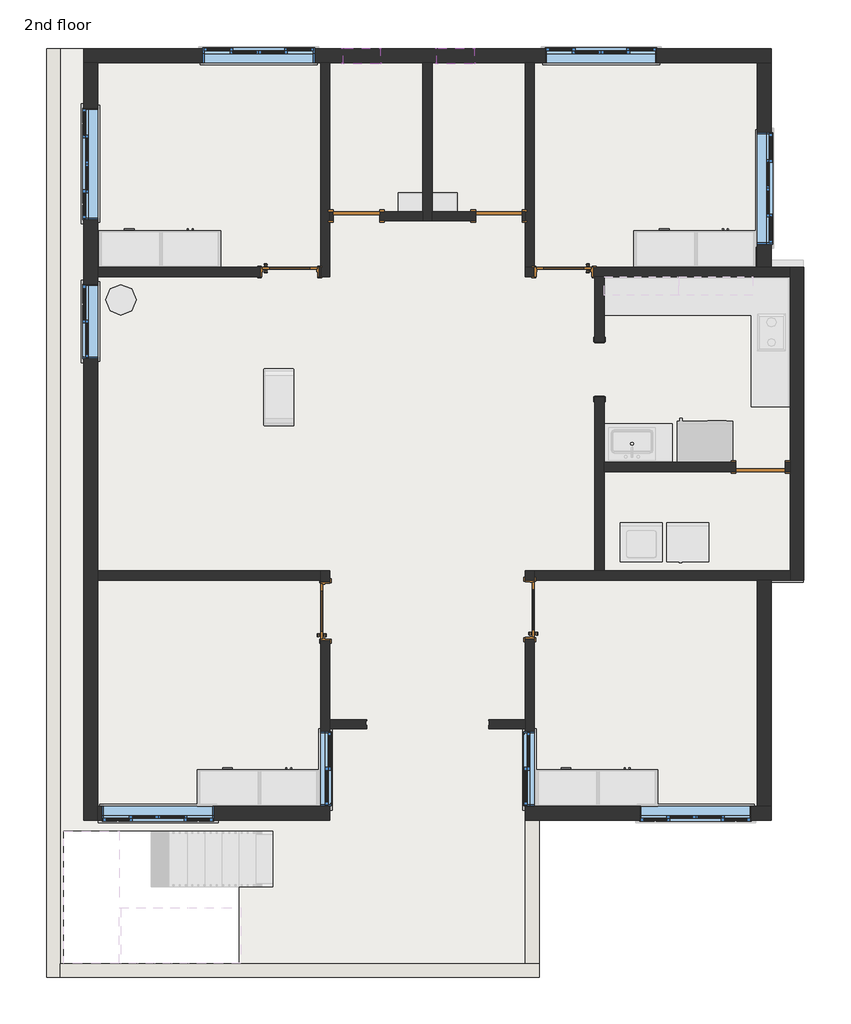
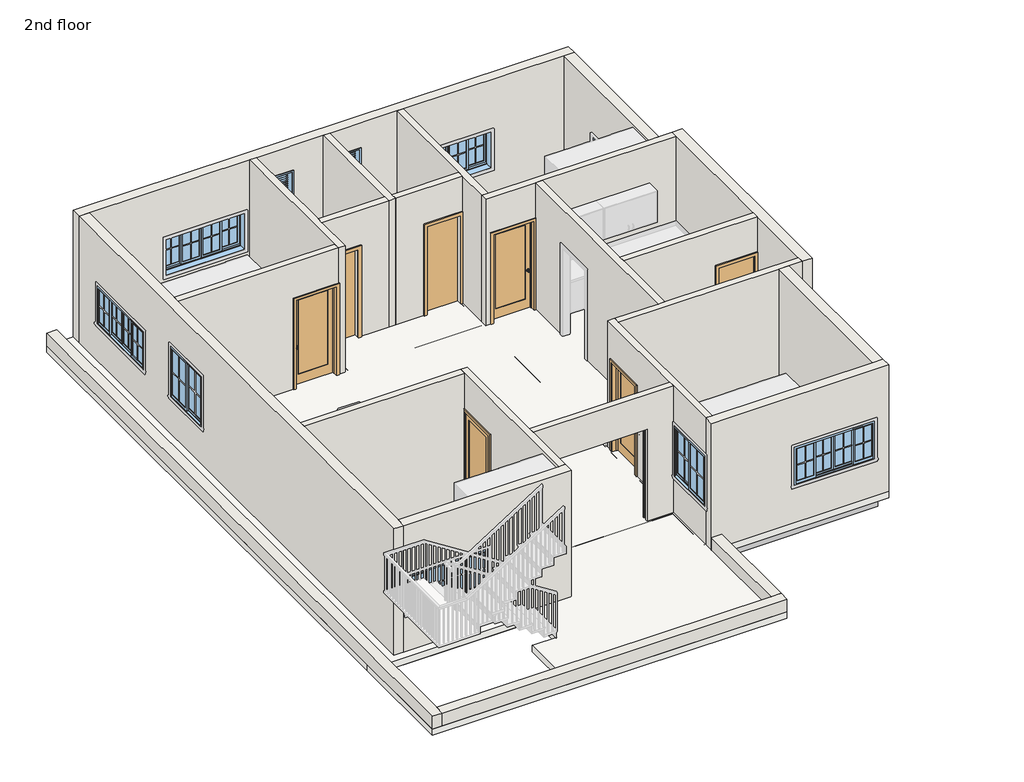
# One storey, part 1 of 4: 24 walls, 11 windows, 7 beams, 7 doors, 1 slab.
"""IFC4 building model written with IfcOpenShell, lengths in millimetres."""

from ifc_helpers import new_model, si_unit, frame, origin, place, context, project, spatial, polyline, outline, extrude, faceted_brep, transform, mapped, element, save
from components import door_010cc4d9, door_5a860750, door_e2b13fe9, door_a9addea7, door_bb092f7c, window_f2d8fef0, window_c1e3dfc0, window_49fe3060, window_58cce754

model = new_model("IFC4")

# Units and contexts
model_context = context("Model", 3, world=origin())
ifc_project = project(units=[si_unit("LENGTHUNIT", "METRE", prefix="MILLI")], contexts=[model_context])

# Site, building, storey
site = spatial("IfcSite", under=ifc_project)
building = spatial("IfcBuilding", under=site)
storey = spatial("IfcBuildingStorey", under=building, Name="2nd floor", Elevation=7010.4)

# Beams
placement = place(None, origin())
element("IfcBeam", 1, ObjectType="Concrete-Rectangular Beam", at=placement, inside=storey, context=model_context, shape_type="SweptSolid", body=[
    extrude(outline(polyline([(-1593.2124084, 1316.1961804), (-1364.6124084, 1316.1961804), (-1364.6124084, -2163.6038196), (-1593.2124084, -2163.6038196), (-1593.2124084, 1316.1961804)])), frame((0.0, 0.0, 6705.6), z_axis=(0.0, 0.0, 1.0), x_axis=(1.0, 0.0, 0.0)), (0.0, 0.0, 1.0), 304.8),
])
element("IfcBeam", 2, ObjectType="Concrete-Rectangular Beam", at=placement, inside=storey, context=model_context, shape_type="Brep", body=[
    faceted_brep([(-1593.2124084, -2201.7038196, 7010.4), (-5212.7124084, -2201.7038196, 7010.4), (-5441.3124084, -2201.7038196, 7010.4), (-5441.3124084, -2239.8038196, 7010.4), (-5174.6124084, -2239.8038196, 7010.4), (-5174.6124084, -2430.3038196, 7010.4), (-1593.2124084, -2430.3038196, 7010.4), (-1593.2124084, -2201.7038196, 6705.6), (-5212.7124084, -2201.7038196, 6705.6), (-5441.3124084, -2201.7038196, 6705.6), (-1593.2124084, -2430.3038196, 6705.6), (-5174.6124084, -2430.3038196, 6705.6), (-5174.6124084, -2239.8038196, 6705.6), (-5441.3124084, -2239.8038196, 6705.6)], [[[0, 1, 2, 3, 4, 5, 6]], [[0, 7, 8, 9, 2, 1]], [[9, 8, 7, 10, 11, 12, 13]], [[10, 6, 5, 11]], [[7, 0, 6, 10]], [[2, 9, 13, 3]], [[12, 4, 3, 13]], [[4, 12, 11, 5]]]),
])
element("IfcBeam", 3, ObjectType="Concrete-Rectangular Beam", at=placement, inside=storey, context=model_context, shape_type="Brep", body=[
    faceted_brep([(-8756.0124084, -2468.4038196, 7010.4), (-8756.0124084, -2239.8038196, 7010.4), (-8794.1124084, -2239.8038196, 7010.4), (-12413.6124084, -2239.8038196, 7010.4), (-12413.6124084, -2468.4038196, 7010.4), (-8756.0124084, -2239.8038196, 6705.6), (-8794.1124084, -2239.8038196, 6705.6), (-12413.6124084, -2239.8038196, 6705.6), (-8756.0124084, -2468.4038196, 6705.6), (-12413.6124084, -2468.4038196, 6705.6)], [[[0, 1, 2, 3, 4]], [[1, 5, 6, 7, 3, 2]], [[5, 8, 9, 7, 6]], [[8, 0, 4, 9]], [[1, 0, 8, 5]], [[4, 3, 7, 9]]]),
])
element("IfcBeam", 4, ObjectType="Concrete-Rectangular Beam", at=placement, inside=storey, context=model_context, shape_type="SweptSolid", body=[
    extrude(outline(polyline([(-12642.2124084, 9875.9961804), (-12413.6124084, 9875.9961804), (-12413.6124084, 6751.7961804), (-12642.2124084, 6751.7961804), (-12642.2124084, 9875.9961804)])), frame((0.0, 0.0, 6705.6), z_axis=(0.0, 0.0, 1.0), x_axis=(1.0, 0.0, 0.0)), (0.0, 0.0, 1.0), 304.8),
    extrude(outline(polyline([(-12413.6124084, -2163.6038196), (-12642.2124084, -2163.6038196), (-12642.2124084, 1392.3961804), (-12413.6124084, 1392.3961804), (-12413.6124084, -2163.6038196)])), frame((0.0, 0.0, 6705.6), z_axis=(0.0, 0.0, 1.0), x_axis=(1.0, 0.0, 0.0)), (0.0, 0.0, 1.0), 304.8),
    extrude(outline(polyline([(-12413.6124084, 1697.1961804), (-12642.2124084, 1697.1961804), (-12642.2124084, 6446.9961804), (-12413.6124084, 6446.9961804), (-12413.6124084, 1697.1961804)])), frame((0.0, 0.0, 6705.6), z_axis=(0.0, 0.0, 1.0), x_axis=(1.0, 0.0, 0.0)), (0.0, 0.0, 1.0), 304.8),
])
element("IfcBeam", 5, ObjectType="Concrete-Rectangular Beam", at=placement, inside=storey, context=model_context, shape_type="Brep", body=[
    faceted_brep([(-843.9124084, 1659.0961804, 7010.4), (-843.9124084, 1430.4961804, 7010.4), (-843.9124084, 1430.4961804, 6705.6), (-843.9124084, 1659.0961804, 6705.6), (-5098.4124084, 1659.0961804, 7010.4), (-5098.4124084, 1468.5961804, 7010.4), (-5403.2124084, 1468.5961804, 7010.4), (-5403.2124084, 1659.0961804, 7010.4), (-5441.3124084, 1659.0961804, 7010.4), (-8565.5124084, 1659.0961804, 7010.4), (-8603.6124084, 1659.0961804, 7010.4), (-8603.6124084, 1468.5961804, 7010.4), (-8908.4124084, 1468.5961804, 7010.4), (-8908.4124084, 1659.0961804, 7010.4), (-12413.6124084, 1659.0961804, 7010.4), (-12413.6124084, 1430.4961804, 7010.4), (-8794.1124084, 1430.4961804, 7010.4), (-8565.5124084, 1430.4961804, 7010.4), (-5441.3124084, 1430.4961804, 7010.4), (-5212.7124084, 1430.4961804, 7010.4), (-1593.2124084, 1430.4961804, 7010.4), (-1593.2124084, 1620.9961804, 7010.4), (-1364.6124084, 1620.9961804, 7010.4), (-1364.6124084, 1430.4961804, 7010.4), (-1364.6124084, 1430.4961804, 6705.6), (-1364.6124084, 1620.9961804, 6705.6), (-1593.2124084, 1620.9961804, 6705.6), (-1593.2124084, 1430.4961804, 6705.6), (-5212.7124084, 1430.4961804, 6705.6), (-5441.3124084, 1430.4961804, 6705.6), (-8565.5124084, 1430.4961804, 6705.6), (-8794.1124084, 1430.4961804, 6705.6), (-12413.6124084, 1430.4961804, 6705.6), (-12413.6124084, 1659.0961804, 6705.6), (-8908.4124084, 1659.0961804, 6705.6), (-8908.4124084, 1468.5961804, 6705.6), (-8603.6124084, 1468.5961804, 6705.6), (-8603.6124084, 1659.0961804, 6705.6), (-8565.5124084, 1659.0961804, 6705.6), (-5441.3124084, 1659.0961804, 6705.6), (-5403.2124084, 1659.0961804, 6705.6), (-5403.2124084, 1468.5961804, 6705.6), (-5098.4124084, 1468.5961804, 6705.6), (-5098.4124084, 1659.0961804, 6705.6)], [[[0, 1, 2, 3]], [[1, 0, 4, 5, 6, 7, 8, 9, 10, 11, 12, 13, 14, 15, 16, 17, 18, 19, 20, 21, 22, 23]], [[2, 1, 23, 24]], [[3, 2, 24, 25, 26, 27, 28, 29, 30, 31, 32, 33, 34, 35, 36, 37, 38, 39, 40, 41, 42, 43]], [[0, 3, 43, 4]], [[15, 14, 33, 32]], [[22, 25, 24, 23]], [[26, 21, 20, 27]], [[21, 26, 25, 22]], [[15, 32, 31, 30, 29, 28, 27, 20, 19, 18, 17, 16]], [[36, 11, 10, 37]], [[11, 36, 35, 12]], [[12, 35, 34, 13]], [[33, 14, 13, 34]], [[42, 5, 4, 43]], [[5, 42, 41, 6]], [[6, 41, 40, 7]], [[37, 10, 9, 8, 7, 40, 39, 38]]]),
])
element("IfcBeam", 6, ObjectType="Concrete-Rectangular Beam", at=placement, inside=storey, context=model_context, shape_type="Brep", body=[
    faceted_brep([(-8794.1124084, -2239.8038196, 7010.4), (-8756.0124084, -2239.8038196, 7010.4), (-8565.5124084, -2239.8038196, 7010.4), (-8565.5124084, -1007.9038196, 7010.4), (-8565.5124084, -779.3038196, 7010.4), (-8565.5124084, 1430.4961804, 7010.4), (-8794.1124084, 1430.4961804, 7010.4), (-8794.1124084, -2239.8038196, 6705.6), (-8794.1124084, 1430.4961804, 6705.6), (-8565.5124084, -2239.8038196, 6705.6), (-8756.0124084, -2239.8038196, 6705.6), (-8565.5124084, 1430.4961804, 6705.6), (-8565.5124084, -779.3038196, 6705.6), (-8565.5124084, -1007.9038196, 6705.6)], [[[0, 1, 2, 3, 4, 5, 6]], [[7, 0, 6, 8]], [[9, 10, 7, 8, 11, 12, 13]], [[11, 5, 4, 3, 2, 9, 13, 12]], [[2, 1, 0, 7, 10, 9]], [[5, 11, 8, 6]]]),
    faceted_brep([(-8794.1124084, 9914.0961804, 7010.4), (-8565.5124084, 9914.0961804, 7010.4), (-8565.5124084, 9914.0961804, 6705.6), (-8794.1124084, 9914.0961804, 6705.6), (-8794.1124084, 6713.6961804, 7010.4), (-8794.1124084, 6713.6961804, 6705.6), (-8756.0124084, 6713.6961804, 6705.6), (-8756.0124084, 6713.6961804, 7010.4), (-8756.0124084, 6751.7961804, 7010.4), (-8565.5124084, 6751.7961804, 7010.4), (-8565.5124084, 7323.2961804, 7010.4), (-8565.5124084, 7551.8961804, 7010.4), (-8565.5124084, 7551.8961804, 6705.6), (-8565.5124084, 7323.2961804, 6705.6), (-8565.5124084, 6751.7961804, 6705.6), (-8756.0124084, 6751.7961804, 6705.6)], [[[0, 1, 2, 3]], [[4, 5, 6, 7]], [[1, 0, 4, 7, 8, 9, 10, 11]], [[3, 2, 12, 13, 14, 15, 6, 5]], [[0, 3, 5, 4]], [[2, 1, 11, 10, 9, 14, 13, 12]], [[15, 8, 7, 6]], [[8, 15, 14, 9]]]),
    faceted_brep([(-8794.1124084, 6485.0961804, 6705.6), (-8794.1124084, 6485.0961804, 7010.4), (-8756.0124084, 6485.0961804, 7010.4), (-8756.0124084, 6485.0961804, 6705.6), (-8565.5124084, 1659.0961804, 6705.6), (-8565.5124084, 1659.0961804, 7010.4), (-8603.6124084, 1659.0961804, 7010.4), (-8603.6124084, 1659.0961804, 6705.6), (-8565.5124084, 6446.9961804, 6705.6), (-8565.5124084, 6446.9961804, 7010.4), (-8794.1124084, 1697.1961804, 7010.4), (-8603.6124084, 1697.1961804, 7010.4), (-8756.0124084, 6446.9961804, 7010.4), (-8794.1124084, 1697.1961804, 6705.6), (-8603.6124084, 1697.1961804, 6705.6), (-8756.0124084, 6446.9961804, 6705.6)], [[[0, 1, 2, 3]], [[4, 5, 6, 7]], [[5, 4, 8, 9]], [[2, 1, 10, 11, 6, 5, 9, 12]], [[1, 0, 13, 10]], [[8, 4, 7, 14, 13, 0, 3, 15]], [[15, 12, 9, 8]], [[12, 15, 3, 2]], [[14, 11, 10, 13]], [[11, 14, 7, 6]]]),
])
element("IfcBeam", 7, ObjectType="Concrete-Rectangular Beam", at=placement, inside=storey, context=model_context, shape_type="SweptSolid", body=[
    extrude(outline(polyline([(-5441.3124084, -779.3038196), (-5441.3124084, -1007.9038196), (-8565.5124084, -1007.9038196), (-8565.5124084, -779.3038196), (-5441.3124084, -779.3038196)])), frame((0.0, 0.0, 6705.6), z_axis=(0.0, 0.0, 1.0), x_axis=(1.0, 0.0, 0.0)), (0.0, 0.0, 1.0), 304.8),
])

# Doors
door_shape = door_010cc4d9(model_context)
element("IfcDoor", 8, ObjectType="Door-Interior-Single-1_Panel-Wood : 36\" x 84\"", at=placement, inside=storey, context=model_context, shape_type="MappedRepresentation", body=[
    mapped(door_shape, transform((-9264.0124084, 6526.3711804, 7010.4), x_axis=(1.0, 0.0, 0.0), y_axis=(0.0, 1.0, 0.0), z_axis=(0.0, 0.0, 1.0))),
])
element("IfcDoor", 9, ObjectType="Door-Interior-Single-1_Panel-Wood : 36\" x 84\"", at=placement, inside=storey, context=model_context, shape_type="MappedRepresentation", body=[
    mapped(door_shape, transform((-8682.9874084, 960.5961804, 7010.4), x_axis=(0.0, 1.0, 0.0), y_axis=(-1.0, 0.0, 0.0), z_axis=(0.0, 0.0, 1.0))),
])
door_2_shape = door_5a860750(model_context)
element("IfcDoor", 10, ObjectType="Door-Interior-Single-1_Panel-Wood : 36\" x 84\"", at=placement, inside=storey, context=model_context, shape_type="MappedRepresentation", body=[
    mapped(door_2_shape, transform((-4768.2124084, 6526.3711804, 7010.4), x_axis=(-1.0, 0.0, 0.0), y_axis=(0.0, -1.0, 0.0), z_axis=(0.0, 0.0, 1.0))),
])
element("IfcDoor", 11, ObjectType="Door-Interior-Single-1_Panel-Wood : 36\" x 84\"", at=placement, inside=storey, context=model_context, shape_type="MappedRepresentation", body=[
    mapped(door_2_shape, transform((-5323.8374084, 985.9961804, 7010.4), x_axis=(0.0, 1.0, 0.0), y_axis=(-1.0, 0.0, 0.0), z_axis=(0.0, 0.0, 1.0))),
])
door_3_shape = door_e2b13fe9(model_context)
element("IfcDoor", 12, ObjectType="Single-Flush : 30\" x 84\"", at=placement, inside=storey, context=model_context, shape_type="MappedRepresentation", body=[
    mapped(door_3_shape, transform((-8171.8124084, 7437.5961804, 7010.4), x_axis=(-1.0, 0.0, 0.0), y_axis=(0.0, -1.0, 0.0), z_axis=(0.0, 0.0, 1.0))),
])
door_4_shape = door_a9addea7(model_context)
element("IfcDoor", 13, ObjectType="Single-Flush : 30\" x 84\"", at=placement, inside=storey, context=model_context, shape_type="MappedRepresentation", body=[
    mapped(door_4_shape, transform((-5835.0124084, 7437.5961804, 7010.4), x_axis=(1.0, 0.0, 0.0), y_axis=(0.0, 1.0, 0.0), z_axis=(0.0, 0.0, 1.0))),
])
door_5_shape = door_bb092f7c(model_context)
element("IfcDoor", 14, ObjectType="Single-Flush : 32\" x 84\"", at=placement, inside=storey, context=model_context, shape_type="MappedRepresentation", body=[
    mapped(door_5_shape, transform((-1542.4124084, 3322.7961804, 7010.4), x_axis=(1.0, 0.0, 0.0), y_axis=(0.0, 1.0, 0.0), z_axis=(0.0, 0.0, 1.0))),
])

# Slab
element("IfcSlab", 15, ObjectType="Generic - 6\"", at=placement, inside=storey, context=model_context, shape_type="SweptSolid", body=[
    extrude(outline(polyline([(-1364.6124084, 10180.7961804), (-1364.6124084, 6599.3961804), (-831.2124084, 6599.3961804), (-831.2124084, 1468.5961804), (-1364.6124084, 1468.5961804), (-1364.6124084, -2468.4038196), (-5174.6124084, -2468.4038196), (-5174.6124084, -5046.5038196), (-13251.8124084, -5046.5038196), (-13251.8124084, -2468.4038196), (-13251.8124084, 10180.7961804), (-1364.6124084, 10180.7961804)]), holes=[polyline([(-9543.8120641, -3536.9669819), (-9543.8120641, -2647.9669819), (-12972.8120641, -2647.9669819), (-12972.8120641, -4817.9038196), (-10102.6120641, -4817.9038196), (-10102.6120641, -3536.9669819), (-9543.8120641, -3536.9669819)])]), frame((0.0, 0.0, 6858.0), z_axis=(0.0, 0.0, 1.0), x_axis=(1.0, 0.0, 0.0)), (0.0, 0.0, 1.0), 152.4),
])

# Walls
element("IfcWall", 16, ObjectType="Generic - 6\"", at=placement, inside=storey, context=model_context, shape_type="Brep", body=[
    faceted_brep([(-8756.0124084, 9952.1961804, 7010.4), (-8756.0124084, 6599.3961804, 7010.4), (-8756.0124084, 6446.9961804, 7010.4), (-8756.0124084, 6446.9961804, 10058.4), (-8756.0124084, 6599.3961804, 10058.4), (-8756.0124084, 9952.1961804, 10058.4), (-8603.6124084, 9952.1961804, 7010.4), (-8603.6124084, 9952.1961804, 10058.4), (-8603.6124084, 7513.7961804, 10058.4), (-8603.6124084, 7361.3961804, 10058.4), (-8603.6124084, 6446.9961804, 10058.4), (-8603.6124084, 6446.9961804, 7010.4), (-8603.6124084, 7361.3961804, 7010.4), (-8603.6124084, 7513.7961804, 7010.4)], [[[0, 1, 2, 3, 4, 5]], [[6, 7, 8, 9, 10, 11, 12, 13]], [[2, 1, 0, 6, 13, 12, 11]], [[0, 5, 7, 6]], [[3, 2, 11, 10]], [[5, 4, 3, 10, 9, 8, 7]]]),
])
element("IfcWall", 17, ObjectType="Generic - 6\"", at=placement, inside=storey, context=model_context, shape_type="SweptSolid", body=[
    extrude(outline(polyline([(7010.4, -8756.0124084), (10058.4, -8756.0124084), (10058.4, -12413.6124084), (7010.4, -12413.6124084), (7010.4, -9746.6124084), (9169.4, -9746.6124084), (9169.4, -8781.4124084), (7010.4, -8781.4124084), (7010.4, -8756.0124084)])), frame((0.0, 6446.9961804, 0.0), z_axis=(0.0, 1.0, 0.0), x_axis=(0.0, 0.0, 1.0)), (0.0, 0.0, 1.0), 152.4),
])
element("IfcWall", 18, ObjectType="Generic - 6\"", at=placement, inside=storey, context=model_context, shape_type="Brep", body=[
    faceted_brep([(-7079.6124084, 9952.1961804, 7010.4), (-7079.6124084, 7513.7961804, 7010.4), (-7079.6124084, 7361.3961804, 7010.4), (-7079.6124084, 7361.3961804, 10058.4), (-7079.6124084, 7513.7961804, 10058.4), (-7079.6124084, 9952.1961804, 10058.4), (-6927.2124084, 9952.1961804, 7010.4), (-6927.2124084, 9952.1961804, 10058.4), (-6927.2124084, 7513.7961804, 10058.4), (-6927.2124084, 7361.3961804, 10058.4), (-6927.2124084, 7361.3961804, 7010.4), (-6927.2124084, 7513.7961804, 7010.4)], [[[0, 1, 2, 3, 4, 5]], [[6, 7, 8, 9, 10, 11]], [[2, 1, 0, 6, 11, 10]], [[0, 5, 7, 6]], [[3, 2, 10, 9]], [[5, 4, 3, 9, 8, 7]]]),
])
element("IfcWall", 19, ObjectType="Generic - 6\"", at=placement, inside=storey, context=model_context, shape_type="SweptSolid", body=[
    extrude(outline(polyline([(7010.4, -7079.6124084), (10058.4, -7079.6124084), (10058.4, -8603.6124084), (7010.4, -8603.6124084), (7010.4, -8552.8124084), (9144.0, -8552.8124084), (9144.0, -7790.8124084), (7010.4, -7790.8124084), (7010.4, -7079.6124084)])), frame((0.0, 7361.3961804, 0.0), z_axis=(0.0, 1.0, 0.0), x_axis=(0.0, 0.0, 1.0)), (0.0, 0.0, 1.0), 152.4),
])
element("IfcWall", 20, ObjectType="Generic - 6\"", at=placement, inside=storey, context=model_context, shape_type="SweptSolid", body=[
    extrude(outline(polyline([(10058.4, -6927.2124084), (7010.4, -6927.2124084), (7010.4, -6216.0124084), (9144.0, -6216.0124084), (9144.0, -5454.0124084), (7010.4, -5454.0124084), (7010.4, -5403.2124084), (10058.4, -5403.2124084), (10058.4, -6927.2124084)])), frame((0.0, 7361.3961804, 0.0), z_axis=(0.0, 1.0, 0.0), x_axis=(0.0, 0.0, 1.0)), (0.0, 0.0, 1.0), 152.4),
])
element("IfcWall", 21, ObjectType="Generic - 6\"", at=placement, inside=storey, context=model_context, shape_type="Brep", body=[
    faceted_brep([(-5250.8124084, 6599.3961804, 7010.4), (-5250.8124084, 9952.1961804, 7010.4), (-5250.8124084, 9952.1961804, 10058.4), (-5250.8124084, 6599.3961804, 10058.4), (-5403.2124084, 6599.3961804, 7010.4), (-5403.2124084, 6599.3961804, 10058.4), (-5403.2124084, 7361.3961804, 10058.4), (-5403.2124084, 7513.7961804, 10058.4), (-5403.2124084, 9952.1961804, 10058.4), (-5403.2124084, 9952.1961804, 7010.4), (-5403.2124084, 7513.7961804, 7010.4), (-5403.2124084, 7361.3961804, 7010.4)], [[[0, 1, 2, 3]], [[4, 5, 6, 7, 8, 9, 10, 11]], [[1, 0, 4, 11, 10, 9]], [[2, 1, 9, 8]], [[0, 3, 5, 4]], [[3, 2, 8, 7, 6, 5]]]),
])
element("IfcWall", 22, ObjectType="Generic - 6\"", at=placement, inside=storey, context=model_context, shape_type="Brep", body=[
    faceted_brep([(-5403.2124084, 6599.3961804, 7010.4), (-5403.2124084, 6599.3961804, 10058.4), (-5250.8124084, 6599.3961804, 10058.4), (-1593.2124084, 6599.3961804, 10058.4), (-1364.6124084, 6599.3961804, 10058.4), (-1059.8124084, 6599.3961804, 10058.4), (-1059.8124084, 6599.3961804, 7010.4), (-1364.6124084, 6599.3961804, 7010.4), (-1593.2124084, 6599.3961804, 7010.4), (-4285.6124084, 6599.3961804, 7010.4), (-4285.6124084, 6599.3961804, 9169.4), (-5250.8124084, 6599.3961804, 9169.4), (-5250.8124084, 6599.3961804, 7010.4), (-1059.8124084, 6446.9961804, 10058.4), (-4107.8124084, 6446.9961804, 10058.4), (-4260.2124084, 6446.9961804, 10058.4), (-5403.2124084, 6446.9961804, 10058.4), (-5403.2124084, 6446.9961804, 7010.4), (-5250.8124084, 6446.9961804, 7010.4), (-5250.8124084, 6446.9961804, 9169.4), (-4285.6124084, 6446.9961804, 9169.4), (-4285.6124084, 6446.9961804, 7010.4), (-4260.2124084, 6446.9961804, 7010.4), (-4107.8124084, 6446.9961804, 7010.4), (-1059.8124084, 6446.9961804, 7010.4)], [[[0, 1, 2, 3, 4, 5, 6, 7, 8, 9, 10, 11, 12]], [[13, 14, 15, 16, 17, 18, 19, 20, 21, 22, 23, 24]], [[17, 0, 12, 18]], [[6, 24, 23, 22, 21, 9, 8, 7]], [[1, 0, 17, 16]], [[6, 5, 13, 24]], [[11, 19, 18, 12]], [[19, 11, 10, 20]], [[20, 10, 9, 21]], [[16, 15, 14, 13, 5, 4, 3, 2, 1]]]),
])
element("IfcWall", 23, ObjectType="Generic - 6\"", at=placement, inside=storey, context=model_context, shape_type="SweptSolid", body=[
    extrude(outline(polyline([(-8756.0124084, 1468.5961804), (-12413.6124084, 1468.5961804), (-12413.6124084, 1620.9961804), (-8756.0124084, 1620.9961804), (-8756.0124084, 1468.5961804)])), frame((0.0, 0.0, 7010.4), z_axis=(0.0, 0.0, 1.0), x_axis=(1.0, 0.0, 0.0)), (0.0, 0.0, 1.0), 3048.0),
])
element("IfcWall", 24, ObjectType="Generic - 6\"", at=placement, inside=storey, context=model_context, shape_type="Brep", body=[
    faceted_brep([(-5403.2124084, -2239.8038196, 7010.4), (-5403.2124084, -2239.8038196, 10058.4), (-5403.2124084, -969.8038196, 10058.4), (-5403.2124084, -817.4038196, 10058.4), (-5403.2124084, 1620.9961804, 10058.4), (-5403.2124084, 1620.9961804, 7010.4), (-5403.2124084, 1468.5961804, 7010.4), (-5403.2124084, 1468.5961804, 9169.4), (-5403.2124084, 503.3961804, 9169.4), (-5403.2124084, 503.3961804, 7010.4), (-5403.2124084, -817.4038196, 7010.4), (-5403.2124084, -969.8038196, 7010.4), (-5403.2124084, -1014.2538196, 7924.8), (-5403.2124084, -1014.2538196, 9144.0), (-5403.2124084, -2233.4538196, 9144.0), (-5403.2124084, -2233.4538196, 7924.8), (-5250.8124084, -2239.8038196, 10058.4), (-5250.8124084, -2239.8038196, 7010.4), (-5250.8124084, 503.3961804, 7010.4), (-5250.8124084, 503.3961804, 9169.4), (-5250.8124084, 1468.5961804, 9169.4), (-5250.8124084, 1468.5961804, 7010.4), (-5250.8124084, 1620.9961804, 7010.4), (-5250.8124084, 1620.9961804, 10058.4), (-5250.8124084, 1468.5961804, 10058.4), (-5250.8124084, -1014.2538196, 9144.0), (-5250.8124084, -1014.2538196, 7924.8), (-5250.8124084, -2233.4538196, 7924.8), (-5250.8124084, -2233.4538196, 9144.0)], [[[0, 1, 2, 3, 4, 5, 6, 7, 8, 9, 10, 11], [12, 13, 14, 15]], [[16, 17, 18, 19, 20, 21, 22, 23, 24], [25, 26, 27, 28]], [[17, 0, 11, 10, 9, 18]], [[5, 22, 21, 6]], [[1, 0, 17, 16]], [[5, 4, 23, 22]], [[20, 7, 6, 21]], [[7, 20, 19, 8]], [[8, 19, 18, 9]], [[25, 13, 12, 26]], [[26, 12, 15, 27]], [[27, 15, 14, 28]], [[13, 25, 28, 14]], [[4, 3, 2, 1, 16, 24, 23]]]),
])
element("IfcWall", 25, ObjectType="Generic - 6\"", at=placement, inside=storey, context=model_context, shape_type="Brep", body=[
    faceted_brep([(-8756.0124084, 1620.9961804, 7010.4), (-8756.0124084, 1468.5961804, 7010.4), (-8756.0124084, 1443.1961804, 7010.4), (-8756.0124084, 1443.1961804, 9169.4), (-8756.0124084, 477.9961804, 9169.4), (-8756.0124084, 477.9961804, 7010.4), (-8756.0124084, -2239.8038196, 7010.4), (-8756.0124084, -2239.8038196, 10058.4), (-8756.0124084, 1468.5961804, 10058.4), (-8756.0124084, 1620.9961804, 10058.4), (-8756.0124084, -2233.4538196, 9144.0), (-8756.0124084, -2233.4538196, 7924.8), (-8756.0124084, -1014.2538196, 7924.8), (-8756.0124084, -1014.2538196, 9144.0), (-8603.6124084, 1443.1961804, 7010.4), (-8603.6124084, 1620.9961804, 7010.4), (-8603.6124084, 1620.9961804, 10058.4), (-8603.6124084, -817.4038196, 10058.4), (-8603.6124084, -969.8038196, 10058.4), (-8603.6124084, -2239.8038196, 10058.4), (-8603.6124084, -2239.8038196, 7010.4), (-8603.6124084, -969.8038196, 7010.4), (-8603.6124084, -817.4038196, 7010.4), (-8603.6124084, 477.9961804, 7010.4), (-8603.6124084, 477.9961804, 9169.4), (-8603.6124084, 1443.1961804, 9169.4), (-8603.6124084, -2233.4538196, 7924.8), (-8603.6124084, -2233.4538196, 9144.0), (-8603.6124084, -1014.2538196, 9144.0), (-8603.6124084, -1014.2538196, 7924.8)], [[[0, 1, 2, 3, 4, 5, 6, 7, 8, 9], [10, 11, 12, 13]], [[14, 15, 16, 17, 18, 19, 20, 21, 22, 23, 24, 25], [26, 27, 28, 29]], [[6, 5, 23, 22, 21, 20]], [[2, 1, 0, 15, 14]], [[25, 3, 2, 14]], [[3, 25, 24, 4]], [[4, 24, 23, 5]], [[0, 9, 16, 15]], [[10, 27, 26, 11]], [[11, 26, 29, 12]], [[12, 29, 28, 13]], [[27, 10, 13, 28]], [[9, 8, 7, 19, 18, 17, 16]], [[7, 6, 20, 19]]]),
])
element("IfcWall", 26, ObjectType="Generic - 6\"", at=placement, inside=storey, context=model_context, shape_type="Brep", body=[
    faceted_brep([(-4260.2124084, 6446.9961804, 10058.4), (-4260.2124084, 6446.9961804, 7010.4), (-4260.2124084, 5380.1961804, 7010.4), (-4260.2124084, 5380.1961804, 9144.0), (-4260.2124084, 4465.7961804, 9144.0), (-4260.2124084, 4465.7961804, 7010.4), (-4260.2124084, 1620.9961804, 7010.4), (-4260.2124084, 1620.9961804, 10058.4), (-4107.8124084, 6446.9961804, 7010.4), (-4107.8124084, 6446.9961804, 10058.4), (-4107.8124084, 3398.9961804, 10058.4), (-4107.8124084, 3246.5961804, 10058.4), (-4107.8124084, 1620.9961804, 10058.4), (-4107.8124084, 1620.9961804, 7010.4), (-4107.8124084, 3246.5961804, 7010.4), (-4107.8124084, 3398.9961804, 7010.4), (-4107.8124084, 4465.7961804, 7010.4), (-4107.8124084, 4465.7961804, 9144.0), (-4107.8124084, 5380.1961804, 9144.0), (-4107.8124084, 5380.1961804, 7010.4)], [[[0, 1, 2, 3, 4, 5, 6, 7]], [[8, 9, 10, 11, 12, 13, 14, 15, 16, 17, 18, 19]], [[1, 8, 19, 2]], [[13, 6, 5, 16, 15, 14]], [[1, 0, 9, 8]], [[7, 6, 13, 12]], [[4, 17, 16, 5]], [[18, 3, 2, 19]], [[17, 4, 3, 18]], [[0, 7, 12, 11, 10, 9]]]),
])
element("IfcWall", 27, ObjectType="Generic - 6\"", at=placement, inside=storey, context=model_context, shape_type="SweptSolid", body=[
    extrude(outline(polyline([(10058.4, -4107.8124084), (7010.4, -4107.8124084), (7010.4, -1948.8124084), (9144.0, -1948.8124084), (9144.0, -1136.0124084), (7010.4, -1136.0124084), (7010.4, -1059.8124084), (10058.4, -1059.8124084), (10058.4, -4107.8124084)])), frame((0.0, 3246.5961804, 0.0), z_axis=(0.0, 1.0, 0.0), x_axis=(0.0, 0.0, 1.0)), (0.0, 0.0, 1.0), 152.4),
])
element("IfcWall", 28, ObjectType="Generic - 6\"", at=placement, inside=storey, context=model_context, shape_type="Brep", body=[
    faceted_brep([(-5250.8124084, 1468.5961804, 7010.4), (-1593.2124084, 1468.5961804, 7010.4), (-1364.6124084, 1468.5961804, 7010.4), (-1059.8124084, 1468.5961804, 7010.4), (-1059.8124084, 1468.5961804, 10058.4), (-1364.6124084, 1468.5961804, 10058.4), (-1593.2124084, 1468.5961804, 10058.4), (-5250.8124084, 1468.5961804, 10058.4), (-5250.8124084, 1620.9961804, 7010.4), (-5250.8124084, 1620.9961804, 10058.4), (-4260.2124084, 1620.9961804, 10058.4), (-4107.8124084, 1620.9961804, 10058.4), (-1059.8124084, 1620.9961804, 10058.4), (-1059.8124084, 1620.9961804, 7010.4), (-4107.8124084, 1620.9961804, 7010.4), (-4260.2124084, 1620.9961804, 7010.4)], [[[0, 1, 2, 3, 4, 5, 6, 7]], [[8, 9, 10, 11, 12, 13, 14, 15]], [[3, 2, 1, 0, 8, 15, 14, 13]], [[4, 3, 13, 12]], [[0, 7, 9, 8]], [[7, 6, 5, 4, 12, 11, 10, 9]]]),
])
element("IfcWall", 29, ObjectType="Generic - 6\"", at=placement, inside=storey, context=model_context, shape_type="Brep", body=[
    faceted_brep([(-5403.2124084, -969.8038196, 7010.4), (-5403.2124084, -969.8038196, 10058.4), (-8603.6124084, -969.8038196, 10058.4), (-8603.6124084, -969.8038196, 7010.4), (-8003.4124084, -969.8038196, 7010.4), (-8003.4124084, -969.8038196, 9219.4), (-6003.4124084, -969.8038196, 9219.4), (-6003.4124084, -969.8038196, 7010.4), (-5403.2124084, -817.4038196, 10058.4), (-5403.2124084, -817.4038196, 7010.4), (-6003.4124084, -817.4038196, 7010.4), (-6003.4124084, -817.4038196, 9219.4), (-8003.4124084, -817.4038196, 9219.4), (-8003.4124084, -817.4038196, 7010.4), (-8603.6124084, -817.4038196, 7010.4), (-8603.6124084, -817.4038196, 10058.4), (-8003.4124084, -837.4038196, 7010.4), (-8018.4124084, -837.4038196, 7010.4), (-8018.4124084, -907.4038196, 7010.4), (-8003.4124084, -907.4038196, 7010.4), (-6003.4124084, -907.4038196, 7010.4), (-5988.4124084, -907.4038196, 7010.4), (-5988.4124084, -837.4038196, 7010.4), (-6003.4124084, -837.4038196, 7010.4), (-6003.4124084, -837.4038196, 9219.4), (-8003.4124084, -837.4038196, 9219.4), (-8003.4124084, -907.4038196, 9219.4), (-6003.4124084, -907.4038196, 9219.4), (-8018.4124084, -907.4038196, 9234.4), (-5988.4124084, -907.4038196, 9234.4), (-5988.4124084, -837.4038196, 9234.4), (-8018.4124084, -837.4038196, 9234.4)], [[[0, 1, 2, 3, 4, 5, 6, 7]], [[8, 9, 10, 11, 12, 13, 14, 15]], [[3, 14, 13, 16, 17, 18, 19, 4]], [[9, 0, 7, 20, 21, 22, 23, 10]], [[1, 0, 9, 8]], [[3, 2, 15, 14]], [[24, 25, 12, 11]], [[26, 27, 6, 5]], [[19, 26, 5, 4]], [[27, 20, 7, 6]], [[27, 26, 19, 18, 28, 29, 21, 20]], [[21, 29, 30, 22]], [[25, 24, 23, 22, 30, 31, 17, 16]], [[23, 24, 11, 10]], [[25, 16, 13, 12]], [[28, 18, 17, 31]], [[29, 28, 31, 30]], [[2, 1, 8, 15]]]),
])
element("IfcWall", 30, ObjectType="Generic - 9\"", at=placement, inside=storey, context=model_context, shape_type="Brep", body=[
    faceted_brep([(-12642.2124084, 9952.1961804, 7010.4), (-12413.6124084, 9952.1961804, 7010.4), (-8756.0124084, 9952.1961804, 7010.4), (-8603.6124084, 9952.1961804, 7010.4), (-7079.6124084, 9952.1961804, 7010.4), (-6927.2124084, 9952.1961804, 7010.4), (-5403.2124084, 9952.1961804, 7010.4), (-5250.8124084, 9952.1961804, 7010.4), (-1593.2124084, 9952.1961804, 7010.4), (-1364.6124084, 9952.1961804, 7010.4), (-1364.6124084, 9952.1961804, 10058.4), (-1593.2124084, 9952.1961804, 10058.4), (-5250.8124084, 9952.1961804, 10058.4), (-5403.2124084, 9952.1961804, 10058.4), (-6927.2124084, 9952.1961804, 10058.4), (-7079.6124084, 9952.1961804, 10058.4), (-8603.6124084, 9952.1961804, 10058.4), (-8756.0124084, 9952.1961804, 10058.4), (-12413.6124084, 9952.1961804, 10058.4), (-12642.2124084, 9952.1961804, 10058.4), (-3244.2124084, 9952.1961804, 8839.2), (-3244.2124084, 9952.1961804, 7924.8), (-5073.0124084, 9952.1961804, 7924.8), (-5073.0124084, 9952.1961804, 8839.2), (-8857.6124084, 9952.1961804, 8839.2), (-8857.6124084, 9952.1961804, 7924.8), (-10686.4124084, 9952.1961804, 7924.8), (-10686.4124084, 9952.1961804, 8839.2), (-8387.7124084, 9952.1961804, 8839.2), (-8387.7124084, 9952.1961804, 9448.8), (-7778.1124084, 9952.1961804, 9448.8), (-7778.1124084, 9952.1961804, 8839.2), (-6851.0124084, 9952.1961804, 8839.2), (-6851.0124084, 9952.1961804, 9448.8), (-6241.4124084, 9952.1961804, 9448.8), (-6241.4124084, 9952.1961804, 8839.2), (-1364.6124084, 10180.7961804, 7010.4), (-12642.2124084, 10180.7961804, 7010.4), (-12642.2124084, 10180.7961804, 10058.4), (-1364.6124084, 10180.7961804, 10058.4), (-3244.2124084, 10180.7961804, 7924.8), (-3244.2124084, 10180.7961804, 8839.2), (-5073.0124084, 10180.7961804, 8839.2), (-5073.0124084, 10180.7961804, 7924.8), (-8857.6124084, 10180.7961804, 7924.8), (-8857.6124084, 10180.7961804, 8839.2), (-10686.4124084, 10180.7961804, 8839.2), (-10686.4124084, 10180.7961804, 7924.8), (-8387.7124084, 10180.7961804, 9448.8), (-8387.7124084, 10180.7961804, 8839.2), (-7778.1124084, 10180.7961804, 8839.2), (-7778.1124084, 10180.7961804, 9448.8), (-6851.0124084, 10180.7961804, 9448.8), (-6851.0124084, 10180.7961804, 8839.2), (-6241.4124084, 10180.7961804, 8839.2), (-6241.4124084, 10180.7961804, 9448.8)], [[[0, 1, 2, 3, 4, 5, 6, 7, 8, 9, 10, 11, 12, 13, 14, 15, 16, 17, 18, 19], [20, 21, 22, 23], [24, 25, 26, 27], [28, 29, 30, 31], [32, 33, 34, 35]], [[36, 37, 38, 39], [40, 41, 42, 43], [44, 45, 46, 47], [48, 49, 50, 51], [52, 53, 54, 55]], [[9, 8, 7, 6, 5, 4, 3, 2, 1, 0, 37, 36]], [[0, 19, 38, 37]], [[10, 9, 36, 39]], [[20, 41, 40, 21]], [[21, 40, 43, 22]], [[22, 43, 42, 23]], [[41, 20, 23, 42]], [[24, 45, 44, 25]], [[25, 44, 47, 26]], [[46, 27, 26, 47]], [[45, 24, 27, 46]], [[49, 48, 29, 28]], [[50, 49, 28, 31]], [[51, 50, 31, 30]], [[48, 51, 30, 29]], [[53, 52, 33, 32]], [[54, 53, 32, 35]], [[55, 54, 35, 34]], [[52, 55, 34, 33]], [[19, 18, 17, 16, 15, 14, 13, 12, 11, 10, 39, 38]]]),
])
element("IfcWall", 31, ObjectType="Generic - 9\"", at=placement, inside=storey, context=model_context, shape_type="Brep", body=[
    faceted_brep([(-12642.2124084, 9952.1961804, 7010.4), (-12642.2124084, -2468.4038196, 7010.4), (-12642.2124084, -2468.4038196, 10058.4), (-12642.2124084, 9952.1961804, 10058.4), (-12642.2124084, 5100.7961804, 9144.0), (-12642.2124084, 5100.7961804, 7924.8), (-12642.2124084, 6319.9961804, 7924.8), (-12642.2124084, 6319.9961804, 9144.0), (-12642.2124084, 9209.2461804, 7924.8), (-12642.2124084, 9209.2461804, 8839.2), (-12642.2124084, 7380.4461804, 8839.2), (-12642.2124084, 7380.4461804, 7924.8), (-12413.6124084, -2468.4038196, 7010.4), (-12413.6124084, -2239.8038196, 7010.4), (-12413.6124084, 1468.5961804, 7010.4), (-12413.6124084, 1620.9961804, 7010.4), (-12413.6124084, 6446.9961804, 7010.4), (-12413.6124084, 6599.3961804, 7010.4), (-12413.6124084, 9952.1961804, 7010.4), (-12413.6124084, 9952.1961804, 10058.4), (-12413.6124084, 6599.3961804, 10058.4), (-12413.6124084, 6446.9961804, 10058.4), (-12413.6124084, 1620.9961804, 10058.4), (-12413.6124084, 1468.5961804, 10058.4), (-12413.6124084, -2239.8038196, 10058.4), (-12413.6124084, -2468.4038196, 10058.4), (-12413.6124084, 5100.7961804, 7924.8), (-12413.6124084, 5100.7961804, 9144.0), (-12413.6124084, 6319.9961804, 9144.0), (-12413.6124084, 6319.9961804, 7924.8), (-12413.6124084, 9209.2461804, 8839.2), (-12413.6124084, 9209.2461804, 7924.8), (-12413.6124084, 7380.4461804, 7924.8), (-12413.6124084, 7380.4461804, 8839.2)], [[[0, 1, 2, 3], [4, 5, 6, 7], [8, 9, 10, 11]], [[12, 13, 14, 15, 16, 17, 18, 19, 20, 21, 22, 23, 24, 25], [26, 27, 28, 29], [30, 31, 32, 33]], [[1, 0, 18, 17, 16, 15, 14, 13, 12]], [[0, 3, 19, 18]], [[2, 1, 12, 25]], [[4, 27, 26, 5]], [[5, 26, 29, 6]], [[6, 29, 28, 7]], [[30, 9, 8, 31]], [[31, 8, 11, 32]], [[10, 33, 32, 11]], [[9, 30, 33, 10]], [[27, 4, 7, 28]], [[3, 2, 25, 24, 23, 22, 21, 20, 19]]]),
])
element("IfcWall", 32, ObjectType="Generic - 9\"", at=placement, inside=storey, context=model_context, shape_type="SweptSolid", body=[
    extrude(outline(polyline([(9952.1961804, 7010.4), (6599.3961804, 7010.4), (6599.3961804, 10058.4), (9952.1961804, 10058.4), (9952.1961804, 7010.4)]), holes=[polyline([(6980.3961804, 8839.2), (6980.3961804, 7924.8), (8809.1961804, 7924.8), (8809.1961804, 8839.2), (6980.3961804, 8839.2)])]), frame((-1593.2124084, 0.0, 0.0), z_axis=(1.0, 0.0, 0.0), x_axis=(0.0, 1.0, 0.0)), (0.0, 0.0, 1.0), 228.6),
])
element("IfcWall", 33, ObjectType="Generic - 9\"", at=placement, inside=storey, context=model_context, shape_type="Brep", body=[
    faceted_brep([(-12413.6124084, -2468.4038196, 7010.4), (-8603.6124084, -2468.4038196, 7010.4), (-8603.6124084, -2468.4038196, 10058.4), (-12413.6124084, -2468.4038196, 10058.4), (-12337.4124084, -2468.4038196, 7924.8), (-12337.4124084, -2468.4038196, 8839.2), (-10508.6124084, -2468.4038196, 8839.2), (-10508.6124084, -2468.4038196, 7924.8), (-8603.6124084, -2239.8038196, 7010.4), (-8756.0124084, -2239.8038196, 7010.4), (-12413.6124084, -2239.8038196, 7010.4), (-12413.6124084, -2239.8038196, 10058.4), (-8756.0124084, -2239.8038196, 10058.4), (-8603.6124084, -2239.8038196, 10058.4), (-12337.4124084, -2239.8038196, 8839.2), (-12337.4124084, -2239.8038196, 7924.8), (-10508.6124084, -2239.8038196, 7924.8), (-10508.6124084, -2239.8038196, 8839.2)], [[[0, 1, 2, 3], [4, 5, 6, 7]], [[8, 9, 10, 11, 12, 13], [14, 15, 16, 17]], [[1, 0, 10, 9, 8]], [[0, 3, 11, 10]], [[14, 5, 4, 15]], [[15, 4, 7, 16]], [[16, 7, 6, 17]], [[5, 14, 17, 6]], [[3, 2, 13, 12, 11]], [[2, 1, 8, 13]]]),
])
element("IfcWall", 34, ObjectType="Generic - 9\"", at=placement, inside=storey, context=model_context, shape_type="SweptSolid", body=[
    extrude(outline(polyline([(-1593.2124084, -2239.8038196), (-1593.2124084, 1468.5961804), (-1364.6124084, 1468.5961804), (-1364.6124084, -2239.8038196), (-1593.2124084, -2239.8038196)])), frame((0.0, 0.0, 7010.4), z_axis=(0.0, 0.0, 1.0), x_axis=(1.0, 0.0, 0.0)), (0.0, 0.0, 1.0), 3048.0),
])
element("IfcWall", 35, ObjectType="Generic - 9\"", at=placement, inside=storey, context=model_context, shape_type="Brep", body=[
    faceted_brep([(-1059.8124084, 6599.3961804, 7010.4), (-1059.8124084, 6446.9961804, 7010.4), (-1059.8124084, 3398.9961804, 7010.4), (-1059.8124084, 3246.5961804, 7010.4), (-1059.8124084, 1620.9961804, 7010.4), (-1059.8124084, 1468.5961804, 7010.4), (-1059.8124084, 1468.5961804, 10058.4), (-1059.8124084, 1620.9961804, 10058.4), (-1059.8124084, 3246.5961804, 10058.4), (-1059.8124084, 3398.9961804, 10058.4), (-1059.8124084, 6446.9961804, 10058.4), (-1059.8124084, 6599.3961804, 10058.4), (-831.2124084, 6599.3961804, 7010.4), (-831.2124084, 6599.3961804, 10058.4), (-831.2124084, 1468.5961804, 10058.4), (-831.2124084, 1468.5961804, 7010.4)], [[[0, 1, 2, 3, 4, 5, 6, 7, 8, 9, 10, 11]], [[12, 13, 14, 15]], [[5, 4, 3, 2, 1, 0, 12, 15]], [[0, 11, 13, 12]], [[6, 5, 15, 14]], [[11, 10, 9, 8, 7, 6, 14, 13]]]),
])
element("IfcWall", 36, ObjectType="Generic - 9\"", at=placement, inside=storey, context=model_context, shape_type="Brep", body=[
    faceted_brep([(-5403.2124084, -2468.4038196, 7010.4), (-5174.6124084, -2468.4038196, 7010.4), (-1364.6124084, -2468.4038196, 7010.4), (-1364.6124084, -2468.4038196, 10058.4), (-5174.6124084, -2468.4038196, 10058.4), (-5403.2124084, -2468.4038196, 10058.4), (-5403.2124084, -2468.4038196, 7315.2), (-3523.6124084, -2468.4038196, 7924.8), (-3523.6124084, -2468.4038196, 8839.2), (-1694.8124084, -2468.4038196, 8839.2), (-1694.8124084, -2468.4038196, 7924.8), (-1364.6124084, -2239.8038196, 7010.4), (-1593.2124084, -2239.8038196, 7010.4), (-5250.8124084, -2239.8038196, 7010.4), (-5403.2124084, -2239.8038196, 7010.4), (-5403.2124084, -2239.8038196, 10058.4), (-5250.8124084, -2239.8038196, 10058.4), (-1593.2124084, -2239.8038196, 10058.4), (-1364.6124084, -2239.8038196, 10058.4), (-3523.6124084, -2239.8038196, 8839.2), (-3523.6124084, -2239.8038196, 7924.8), (-1694.8124084, -2239.8038196, 7924.8), (-1694.8124084, -2239.8038196, 8839.2)], [[[0, 1, 2, 3, 4, 5, 6], [7, 8, 9, 10]], [[11, 12, 13, 14, 15, 16, 17, 18], [19, 20, 21, 22]], [[2, 1, 0, 14, 13, 12, 11]], [[3, 2, 11, 18]], [[19, 8, 7, 20]], [[20, 7, 10, 21]], [[21, 10, 9, 22]], [[8, 19, 22, 9]], [[18, 17, 16, 15, 5, 4, 3]], [[0, 6, 5, 15, 14]]]),
])
element("IfcWall", 37, ObjectType="Generic - 9\"", at=placement, inside=storey, context=model_context, shape_type="Brep", body=[
    faceted_brep([(-13251.8124084, 10180.7961804, 7010.4), (-13251.8124084, -5046.5038196, 7010.4), (-13251.8124084, -5046.5038196, 7315.2), (-13251.8124084, 10180.7961804, 7315.2), (-13023.2124084, 10180.7961804, 7010.4), (-13023.2124084, 10180.7961804, 7315.2), (-13023.2124084, -4817.9038196, 7315.2), (-13023.2124084, -5046.5038196, 7315.2), (-13023.2124084, -5046.5038196, 7010.4), (-13023.2124084, -4817.9038196, 7010.4)], [[[0, 1, 2, 3]], [[4, 5, 6, 7, 8, 9]], [[1, 0, 4, 9, 8]], [[3, 2, 7, 6, 5]], [[0, 3, 5, 4]], [[2, 1, 8, 7]]]),
])
element("IfcWall", 38, ObjectType="Generic - 9\"", at=placement, inside=storey, context=model_context, shape_type="Brep", body=[
    faceted_brep([(-13023.2124084, -5046.5038196, 7010.4), (-5174.6124084, -5046.5038196, 7010.4), (-5174.6124084, -5046.5038196, 7315.2), (-13023.2124084, -5046.5038196, 7315.2), (-13023.2124084, -4817.9038196, 7010.4), (-13023.2124084, -4817.9038196, 7315.2), (-5403.2124084, -4817.9038196, 7315.2), (-5174.6124084, -4817.9038196, 7315.2), (-5174.6124084, -4817.9038196, 7010.4), (-5403.2124084, -4817.9038196, 7010.4)], [[[0, 1, 2, 3]], [[4, 5, 6, 7, 8, 9]], [[1, 0, 4, 9, 8]], [[3, 2, 7, 6, 5]], [[0, 3, 5, 4]], [[2, 1, 8, 7]]]),
])
element("IfcWall", 39, ObjectType="Generic - 9\"", at=placement, inside=storey, context=model_context, shape_type="SweptSolid", body=[
    extrude(outline(polyline([(-5174.6124084, -2468.4038196), (-5174.6124084, -4817.9038196), (-5403.2124084, -4817.9038196), (-5403.2124084, -2468.4038196), (-5174.6124084, -2468.4038196)])), frame((0.0, 0.0, 7010.4), z_axis=(0.0, 0.0, 1.0), x_axis=(1.0, 0.0, 0.0)), (0.0, 0.0, 1.0), 304.8),
])

# Windows
window_shape = window_f2d8fef0(model_context)
element("IfcWindow", 40, ObjectType="Window-Louvers : 24\" x 24\"", at=placement, inside=storey, context=model_context, shape_type="MappedRepresentation", body=[
    mapped(window_shape, transform((-8082.9124084, 10072.8461804, 7924.8), x_axis=(1.0, 0.0, 0.0), y_axis=(0.0, 1.0, 0.0), z_axis=(0.0, 0.0, 1.0))),
])
element("IfcWindow", 41, ObjectType="Window-Louvers : 24\" x 24\"", at=placement, inside=storey, context=model_context, shape_type="MappedRepresentation", body=[
    mapped(window_shape, transform((-6546.2124084, 10072.8461804, 7924.8), x_axis=(1.0, 0.0, 0.0), y_axis=(0.0, 1.0, 0.0), z_axis=(0.0, 0.0, 1.0))),
])
window_2_shape = window_c1e3dfc0(model_context)
element("IfcWindow", 42, ObjectType="Window-Sliding-Double : 48\" x 48\"", at=placement, inside=storey, context=model_context, shape_type="MappedRepresentation", body=[
    mapped(window_2_shape, transform((-12531.7224084, 5710.3961804, 7010.4), x_axis=(0.0, -1.0, 0.0), y_axis=(1.0, 0.0, 0.0), z_axis=(0.0, 0.0, 1.0))),
])
window_3_shape = window_49fe3060(model_context)
element("IfcWindow", 43, ObjectType="Window-Sliding-Double : 48\" x 48\"", at=placement, inside=storey, context=model_context, shape_type="MappedRepresentation", body=[
    mapped(window_3_shape, transform((-8676.0024084, -1623.8538196, 7010.4), x_axis=(0.0, -1.0, 0.0), y_axis=(1.0, 0.0, 0.0), z_axis=(0.0, 0.0, 1.0))),
])
element("IfcWindow", 44, ObjectType="Window-Sliding-Double : 48\" x 48\"", at=placement, inside=storey, context=model_context, shape_type="MappedRepresentation", body=[
    mapped(window_3_shape, transform((-5330.8224084, -1623.8538196, 7010.4), x_axis=(0.0, 1.0, 0.0), y_axis=(-1.0, 0.0, 0.0), z_axis=(0.0, 0.0, 1.0))),
])
window_4_shape = window_58cce754(model_context)
element("IfcWindow", 45, ObjectType="Window-Sliding-Four : 72\" x 36\"", at=placement, inside=storey, context=model_context, shape_type="MappedRepresentation", body=[
    mapped(window_4_shape, transform((-9772.0124084, 10070.3061804, 7010.4), x_axis=(1.0, 0.0, 0.0), y_axis=(0.0, 1.0, 0.0), z_axis=(0.0, 0.0, 1.0))),
])
element("IfcWindow", 46, ObjectType="Window-Sliding-Four : 72\" x 36\"", at=placement, inside=storey, context=model_context, shape_type="MappedRepresentation", body=[
    mapped(window_4_shape, transform((-12531.7224084, 8294.8461804, 7010.4), x_axis=(0.0, 1.0, 0.0), y_axis=(-1.0, 0.0, 0.0), z_axis=(0.0, 0.0, 1.0))),
])
element("IfcWindow", 47, ObjectType="Window-Sliding-Four : 72\" x 36\"", at=placement, inside=storey, context=model_context, shape_type="MappedRepresentation", body=[
    mapped(window_4_shape, transform((-1475.1024084, 7894.7961804, 7010.4), x_axis=(0.0, -1.0, 0.0), y_axis=(1.0, 0.0, 0.0), z_axis=(0.0, 0.0, 1.0))),
])
element("IfcWindow", 48, ObjectType="Window-Sliding-Four : 72\" x 36\"", at=placement, inside=storey, context=model_context, shape_type="MappedRepresentation", body=[
    mapped(window_4_shape, transform((-4158.6124084, 10070.3061804, 7010.4), x_axis=(1.0, 0.0, 0.0), y_axis=(0.0, 1.0, 0.0), z_axis=(0.0, 0.0, 1.0))),
])
element("IfcWindow", 49, ObjectType="Window-Sliding-Four : 72\" x 36\"", at=placement, inside=storey, context=model_context, shape_type="MappedRepresentation", body=[
    mapped(window_4_shape, transform((-2609.2124084, -2357.9138196, 7010.4), x_axis=(-1.0, 0.0, 0.0), y_axis=(0.0, -1.0, 0.0), z_axis=(0.0, 0.0, 1.0))),
])
element("IfcWindow", 50, ObjectType="Window-Sliding-Four : 72\" x 36\"", at=placement, inside=storey, context=model_context, shape_type="MappedRepresentation", body=[
    mapped(window_4_shape, transform((-11423.0124084, -2357.9138196, 7010.4), x_axis=(-1.0, 0.0, 0.0), y_axis=(0.0, -1.0, 0.0), z_axis=(0.0, 0.0, 1.0))),
])

save(model, "model.ifc")

# Revit data of these elements
# Type "Concrete-Rectangular Beam"
#   Assembly Code = "B10"
#   Length [instance default] = 5' - 0"
#   b = 0' - 9"
#   h = 1' - 0"
#   Structural Material [instance default] = Concrete, Cast-in-Place gray
# Type "Door-Interior-Single-1_Panel-Wood : 36\" x 84\""
#   Type Mark = "8"
#   Assembly Code = "C1020300"
#   Analytic Construction = "Wooden"
#   Top Rail = 0' - 4 11/16"
#   Thickness = 0' - 1 3/8"
#   Thermal Resistance (R) = 2.5876 (h·ft²·°F)/BTU
#   Swing Angle [instance default] = 90.00°
#   Stiles = 0' - 4 3/4"
#   Rough Width = 3' - 2"
#   Rough Height = 7' - 1"
#   Height = 7' - 0"
#   Width = 3' - 0"
#   Heat Transfer Coefficient (U) = 0.3865 BTU/(h·ft²·°F)
#   Bottom Rail = 0' - 9 1/8"
#   Trim Material = Cherry
#   Panel Material = Cherry
#   Frame Material = Cherry
#   Door Handle Material = Aluminum
#   Visual Light Transmittance = 0
#   Solar Heat Gain Coefficient = 0
#   Wall Closure = (empty or 0)
#   Function = (empty or 0)
# Type "Single-Flush : 30\" x 84\""
#   Type Mark = "4"
#   Construction Type Id = "MDOOR"
#   Assembly Code = "C1020"
#   Analytic Construction = "Metal"
#   Thickness = 0' - 2"
#   Heat Transfer Coefficient (U) = 0.651978 BTU/(h·ft²·°F)
#   Height = 7' - 0"
#   Trim Projection Ext = 0' - 1"
#   Trim Projection Int = 0' - 1"
#   Trim Width = 0' - 3"
#   Width = 2' - 6"
#   Define Thermal Properties by = 1
#   Define Thermal Properties by = 1
#   Door Material = Door - Panel
#   Frame Material = Door - Frame
#   Visual Light Transmittance = 0
#   Solar Heat Gain Coefficient = 0
#   Function = (empty or 0)
#   Wall Closure = (empty or 0)
# Type "Single-Flush : 32\" x 84\""
#   Type Mark = "3"
#   Construction Type Id = "MDOOR"
#   Assembly Code = "C1020"
#   Analytic Construction = "Metal"
#   Thickness = 0' - 2"
#   Heat Transfer Coefficient (U) = 0.651978 BTU/(h·ft²·°F)
#   Height = 7' - 0"
#   Trim Projection Ext = 0' - 1"
#   Trim Projection Int = 0' - 1"
#   Trim Width = 0' - 3"
#   Width = 2' - 8"
#   Define Thermal Properties by = 1
#   Define Thermal Properties by = 1
#   Door Material = Door - Panel
#   Frame Material = Door - Frame
#   Visual Light Transmittance = 0
#   Solar Heat Gain Coefficient = 0
#   Function = (empty or 0)
#   Wall Closure = (empty or 0)
# Type "Generic - 6\""
#   Assembly Code = "B1010"
#   Function = 0
#   Layers, outside or top first: 0' - 6" no material (function 1)
# Type "Generic - 6\""
#   Assembly Code = "B2010"
#   Layers, outside or top first: 0' - 6" no material (function 1)
# Type "Generic - 9\""
#   Assembly Code = "B2010"
#   Layers, outside or top first: 0' - 9" no material (function 1)
# Type "Window-Louvers : 24\" x 24\""
#   Type Mark = "24"
#   Construction Type Id = "GSP4R"
#   Assembly Code = "B20"
#   Analytic Construction = "1/8 in Pilkington single glazing"
#   Visual Light Transmittance = 0.9
#   Thermal Resistance (R) = 1.53941 (h·ft²·°F)/BTU
#   Solar Heat Gain Coefficient = 0.78
#   Max Height = 1' - 11.74264"
#   Height = 2' - 0"
#   Heat Transfer Coefficient (U) = 0.6496 BTU/(h·ft²·°F)
#   Blade Width [instance default] = 1' - 10 1/2"
#   Blade Vertical Thickness = 0' - 0.35355"
#   Blade Thickness = 0' - 0 1/4"
#   Blade Spacing = 0' - 1 1/2"
#   Blade Height = 0' - 1.85355"
#   Blade Depth = 0' - 3"
#   Blade Angle = 45.00°
#   Default Sill Height = 3' - 0"
#   Trim Projection_Exterior = 0' - 0 1/2"
#   Trim Projection_Interior = 0' - 0 1/2"
#   Trim Width_Exterior = 0' - 1 1/2"
#   Trim Width_Interior = 0' - 1 1/2"
#   Width = 2' - 0"
#   Max Blade Count = 12
#   Define Thermal Properties by = 1
#   Blade Count = 12
#   Frame Material = Birch
#   Louver Material = Birch
#   Trim Exterior Material = Birch
#   Trim Interior Material = Birch
#   Wall Closure = (empty or 0)
# Type "Window-Sliding-Double : 48\" x 48\""
#   Type Mark = "23"
#   Fire Rating = "0.5h"
#   Assembly Code = "B2020100"
#   Analytic Construction = "Double glazing - domestic"
#   Window Inset [instance default] = 0' - 0"
#   Wall Thickness [instance default] = 0' - 6"
#   Visual Light Transmittance = 0.81
#   Thermal Resistance (R) = 1.8146 (h·ft²·°F)/BTU
#   Solar Heat Gain Coefficient = 0.76
#   Muntin Width = 1' - 8 5/8"
#   Muntin Height = 3' - 6 1/4"
#   Interior Wall Closure [instance default] = 0' - 2 3/4"
#   Heat Transfer Coefficient (U) = 0.5511 BTU/(h·ft²·°F)
#   Frame Extension [instance default] = 0' - 0 1/4"
#   Exterior Wall Closure [instance default] = 0' - 1 1/4"
#   Rough Width = 4' - 0 1/2"
#   Rough Height = 4' - 0 1/2"
#   Height = 4' - 0"
#   Extension Jamb [instance default] = 0' - 2 3/4"
#   Default Sill Height = 3' - 0"
#   Width = 4' - 0"
#   Interior Trim Visibility [instance default] = yes
#   Indicator Visibility [instance default] = yes
#   Exterior Trim Visibility [instance default] = yes
#   Muntin Visibility = yes
#   Extension Jamb Visibility [instance default] = yes
#   Muntin Pattern = Muntin Pattern_2x2 : Muntin Pattern_2x2
#   Interior Trim Material = Wood - Stained
#   Interior Trim = Trim-Window-Interior-Flat : Picture Frame
#   Interior Frame Material = Wood - Stained
#   Glass Panel Material = Glass
#   Exterior Trim Material = Clad - White
#   Exterior Trim = Trim-Window-Exterior-Flat : with Sill
#   Exterior Frame Material = Clad - White
#   Wall Closure = (empty or 0)
# Type "Window-Sliding-Four : 72\" x 36\""
#   Type Mark = "20"
#   Fire Rating = "0.5h"
#   Assembly Code = "B2020100"
#   Analytic Construction = "Double glazing - domestic"
#   Window Inset [instance default] = 0' - 0"
#   Wall Thickness [instance default] = 0' - 6"
#   Visual Light Transmittance = 0.81
#   Thermal Resistance (R) = 1.8146 (h·ft²·°F)/BTU
#   Solar Heat Gain Coefficient = 0.76
#   Interior Wall Closure [instance default] = 0' - 2 19/32"
#   Heat Transfer Coefficient (U) = 0.5511 BTU/(h·ft²·°F)
#   Frame Extension [instance default] = 0' - 0 1/4"
#   Exterior Wall Closure [instance default] = 0' - 1 1/4"
#   Rough Width = 6' - 0 1/2"
#   Rough Height = 3' - 0 1/2"
#   Height = 3' - 0"
#   Extension Jamb [instance default] = 0' - 2 3/4"
#   Default Sill Height = 3' - 0"
#   Width = 6' - 0"
#   Middle Muntin Visibility = yes
#   Interior Trim Visibility [instance default] = yes
#   Indicator Visibility [instance default] = yes
#   Exterior Trim Visibility [instance default] = yes
#   Side Muntin Visibility = yes
#   Extension Jamb Visibility [instance default] = yes
#   Interior Trim Material = Wood - Stained
#   Muntin Pattern = Muntin Pattern_2x2 : Muntin Pattern_2x2
#   Interior Trim = Trim-Window-Interior-Flat : Picture Frame
#   Interior Frame Material = Wood - Stained
#   Glass Panel Material = Glass
#   Exterior Trim Material = Clad - White
#   Exterior Trim = Trim-Window-Exterior-Flat : with Sill
#   Exterior Frame Material = Clad - White
#   Wall Closure = (empty or 0)
# Elements 1, 2, 3, 4, 5, 6, 7 (IfcBeam, "Concrete-Rectangular Beam")
#   Structural Material = Concrete, Cast-in-Place gray
#   Phase Created = New Construction
#   Materials on its faces: "Concrete, Cast-in-Place gray"
# Elements 8, 9, 10, 11 (IfcDoor, "Door-Interior-Single-1_Panel-Wood : 36\" x 84\"")
#   Swing Angle = 90.00°
#   Phase Created = New Construction
#   Materials on its faces: "Cherry", "Aluminum"
# Elements 12, 13 (IfcDoor, "Single-Flush : 30\" x 84\"")
#   Phase Created = New Construction
#   Materials on its faces: "Door - Frame", "Door - Panel"
# Element 14 (IfcDoor, "Single-Flush : 32\" x 84\"")
#   Phase Created = New Construction
#   Materials on its faces: "Door - Frame", "Door - Panel"
# Element 15 (IfcSlab, "Generic - 6\"")
#   Height Offset From Level = 0' - 0"
#   Phase Created = New Construction
#   Materials on its faces: "Default Floor"
# Elements 16, 17, 18, 19, 20, 21, 22, 23, 24, 25, 26, 27, 28, 29 (IfcWall, "Generic - 6\"")
#   Top Offset = 0' - 0"
#   Base Offset = 0' - 0"
#   Unconnected Height = 9' - 6"
#   wall height = 10' - 0"
#   Phase Created = New Construction
#   Base Constraint = 2nd floor
#   Materials on its faces: "Default Wall"
# Elements 30, 31, 32, 33, 34, 35, 36 (IfcWall, "Generic - 9\"")
#   Top Offset = 0' - 0"
#   Base Offset = 0' - 0"
#   Unconnected Height = 9' - 6"
#   wall height = 10' - 0"
#   Phase Created = New Construction
#   Base Constraint = 2nd floor
#   Materials on its faces: "Default Wall"
# Elements 37, 38, 39 (IfcWall, "Generic - 9\"")
#   Top Offset = 0' - 0"
#   Base Offset = 0' - 0"
#   Unconnected Height = 1' - 0"
#   wall height = 1' - 0"
#   Phase Created = New Construction
#   Base Constraint = 2nd floor
#   Materials on its faces: "Default Wall"
# Element 40 (IfcWindow, "Window-Louvers : 24\" x 24\"")
#   Mark = "37"
#   Blade Width = 1' - 10 1/2"
#   Phase Created = New Construction
#   Materials on its faces: "Birch"
# Element 41 (IfcWindow, "Window-Louvers : 24\" x 24\"")
#   Mark = "38"
#   Blade Width = 1' - 10 1/2"
#   Phase Created = New Construction
#   Materials on its faces: "Birch"
# Element 42 (IfcWindow, "Window-Sliding-Double : 48\" x 48\"")
#   Mark = "32"
#   Window Inset = 0' - 0"
#   Interior Wall Closure = 0' - 2 3/4"
#   Frame Extension = 0' - 0 1/4"
#   Exterior Wall Closure = 0' - 1 1/4"
#   Interior Trim Visibility = yes
#   Indicator Visibility = yes
#   Exterior Trim Visibility = yes
#   Phase Created = New Construction
#   Materials on its faces: "Wood - Stained", "Glass", "Clad - White"
# Element 43 (IfcWindow, "Window-Sliding-Double : 48\" x 48\"")
#   Mark = "33"
#   Window Inset = 0' - 0"
#   Interior Wall Closure = 0' - 2 3/4"
#   Frame Extension = 0' - 0 1/4"
#   Exterior Wall Closure = 0' - 1 1/4"
#   Interior Trim Visibility = yes
#   Indicator Visibility = yes
#   Exterior Trim Visibility = yes
#   Phase Created = New Construction
#   Materials on its faces: "Wood - Stained", "Glass", "Clad - White"
# Element 44 (IfcWindow, "Window-Sliding-Double : 48\" x 48\"")
#   Mark = "34"
#   Window Inset = 0' - 0"
#   Interior Wall Closure = 0' - 2 3/4"
#   Frame Extension = 0' - 0 1/4"
#   Exterior Wall Closure = 0' - 1 1/4"
#   Interior Trim Visibility = yes
#   Indicator Visibility = yes
#   Exterior Trim Visibility = yes
#   Phase Created = New Construction
#   Materials on its faces: "Wood - Stained", "Glass", "Clad - White"
# Element 45 (IfcWindow, "Window-Sliding-Four : 72\" x 36\"")
#   Mark = "28"
#   Window Inset = 0' - 0"
